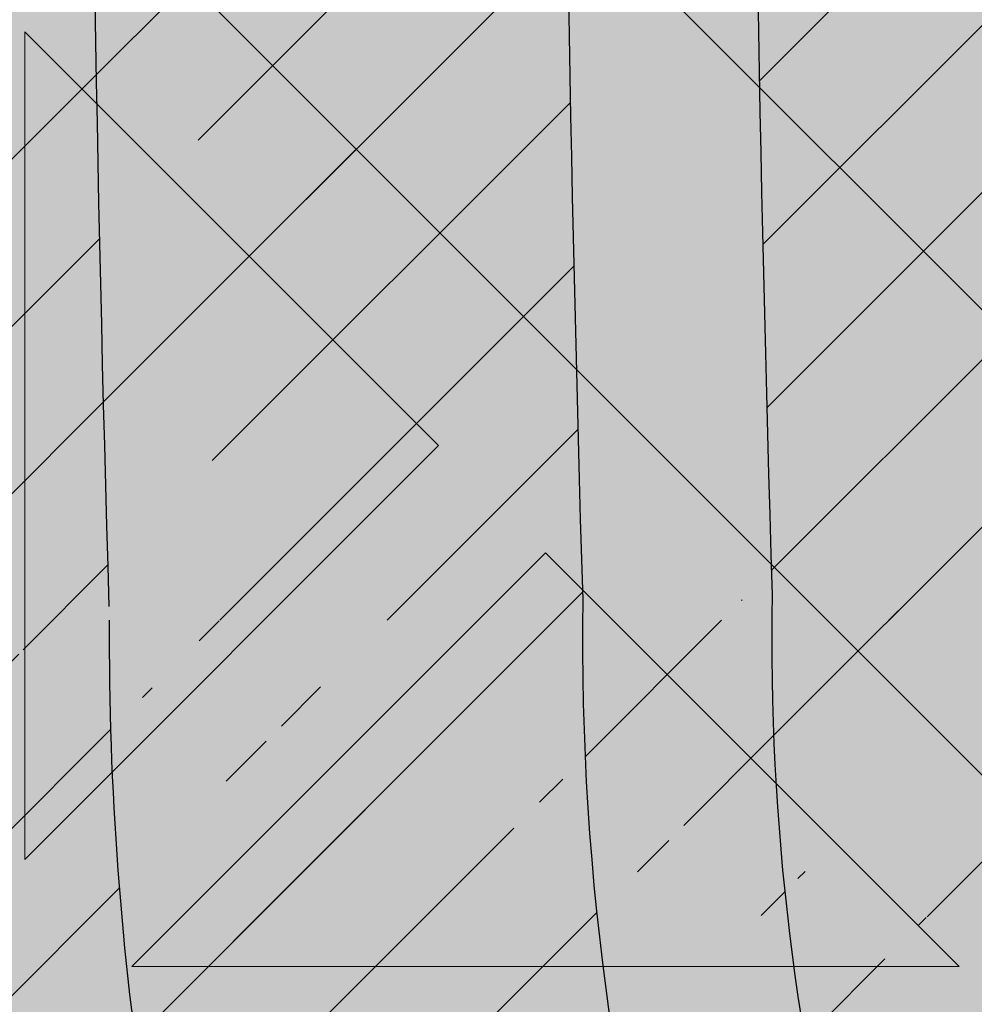
# Model space of a CAD drawing. Units: inches. Extents: x 844 to 2234, y 346 to 1084.
# Tile 11 of 93: x 1120.394 to 1122.002, y 691.183 to 692.842. Entities that reach past the tile are written whole.
import ezdxf

# ---------------------------------------------------------------- set-up
doc = ezdxf.new("R2010")
doc.units = ezdxf.units.IN
doc.header["$MEASUREMENT"] = 0
for name, color, linetype, lineweight in [('A-ANNO-DIMS', 2, 'Continuous', 18), ('furniture', 8, 'Continuous', 18), ('RA-AP-01$0$INT', 35, 'Continuous', 5)]:
    doc.layers.add(name, color=color, linetype=linetype, lineweight=lineweight)
doc.layers.add('RA-AP-01$0$FURN', color=3, linetype='Continuous')
doc.layers.add('RA-AP-01$0$WOOD', color=64, linetype='Continuous')
doc.styles.get("Standard").update_dxf_attribs({"font": 'arial.ttf'})
doc.dimstyles.get("Standard").update_dxf_attribs({"dimtxt": 6, "dimasz": 3, "dimexe": 0.18, "dimexo": 0.0625, "dimgap": 0.09, "dimtad": 0, "dimtih": 1, "dimtoh": 1, "dimdec": 1, "dimzin": 0, "dimdsep": 46, "dimlunit": 3, "dimtxsty": 'Standard', "dimblk": 'ARCHTICK', "dimcen": 0.09, "dimadec": 0, "dimazin": 0, "dimtfac": 1, "dimtdec": 1, "dimtofl": 0, "dimtmove": 0, "dimatfit": 3, "dimfxl": 1, "dimtolj": 1, "dimtzin": 0, "dimarcsym": 0})

# ---------------------------------------------------------------- blocks, each defined once
blk = doc.blocks.new('A$C18D01794')
at = {"layer": 'RA-AP-01$0$INT'}
h = blk.add_hatch(color=256, dxfattribs=at)
h.paths.add_polyline_path([(4.585917135068449, -6.356712009588271), (4.555206456959269, -6.35671200958746), (4.555206456959137, -6.387422687716308), (4.874495778835233, -6.706712009592356), (4.90520645695423, -6.676001331474049)])
h.paths.add_polyline_path([(5.255206456948813, -6.387422687716306), (5.255206456948682, -6.356712009605972), (5.224495778822613, -6.356712009605161), (4.905206456953498, -6.676001331474273), (4.935917135072151, -6.706712009592924)])
h.paths.add_polyline_path([(4.935917135072559, -6.706712009592068), (4.905206456953564, -6.737422687710376), (5.255206456951813, -7.087422687708613), (5.255206456951549, -7.026001331471008)])
h.paths.add_polyline_path([(4.555206456956399, -7.026001331471013), (4.555206456956134, -7.087422687708616), (4.905206456953821, -6.737422687710943), (4.874495778835166, -6.70671200959229)])
h = blk.add_hatch(color=256, dxfattribs=at)
h.paths.add_polyline_path([(4.585917135068448, -6.356712009588273), (4.614201406330596, -6.356712009589021), (4.668846067270487, -6.411356670531338), (4.723490728212344, -6.356712009591912), (4.771774999457151, -6.35671200959319), (4.826419660396886, -6.411356670535356), (4.862780050090322, -6.374996280843536), (4.844495778842715, -6.356712009595112), (4.862780050090411, -6.356712009595595), (4.905206456960182, -6.399138416468211), (4.947632863832445, -6.356712009597838), (4.965917135079675, -6.356712009598322), (4.947632863831759, -6.374996280845421), (4.983993253523576, -6.411356670538857), (5.038637914464627, -6.356712009600247), (5.08692218571208, -6.356712009601523), (5.141566846649976, -6.411356670541852), (5.196211507589851, -6.356712009604411), (5.224495778822615, -6.356712009605161), (4.905206456953975, -6.676001331473793)])
h.paths.add_polyline_path([(4.895206456956031, -6.637717060225675), (4.895206456958921, -6.528427738347902), (4.840561796018589, -6.583072399285802)], flags=16)
h.paths.add_polyline_path([(4.915206456955638, -6.637717060226121), (4.969851117895509, -6.583072399288678), (4.915206456957609, -6.528427738348344)], flags=16)
h.paths.add_polyline_path([(4.826419660395175, -6.568930263661755), (4.881064321335613, -6.514285602723745), (4.771774999456703, -6.514285602720857)], flags=16)
h.paths.add_polyline_path([(4.983993253519558, -6.568930263665262), (5.038637914460456, -6.514285602726792), (4.929348592581548, -6.514285602724816)], flags=16)
h.paths.add_polyline_path([(4.881064321336025, -6.494285602723742), (4.826419660397532, -6.439640941782821), (4.771774999457062, -6.494285602720859)], flags=16)
h.paths.add_polyline_path([(4.929348592582019, -6.494285602724817), (5.038637914460982, -6.494285602726792), (4.983993253522945, -6.439640941786327)], flags=16)
h.paths.add_polyline_path([(4.895206456960191, -6.480143467100443), (4.895206456962115, -6.407422687715913), (4.876922185715016, -6.389138416467584), (4.840561796021581, -6.425498806159401)], flags=16)
h.paths.add_polyline_path([(4.915206456958487, -6.480143467100889), (4.969851117899527, -6.425498806162279), (4.933490728206909, -6.389138416468043), (4.9152064569598, -6.40742268771434)], flags=16)
h.paths.add_polyline_path([(4.757632863832376, -6.480143467096812), (4.812277524772842, -6.425498806158772), (4.757632863834348, -6.370854145217844)], flags=16)
h.paths.add_polyline_path([(4.737632863832376, -6.480143467096286), (4.737632863834348, -6.370854145217375), (4.682988202893906, -6.425498806155385)], flags=16)
h.paths.add_polyline_path([(5.05278005008503, -6.480143467103376), (5.052780050087917, -6.370854145224413), (4.998135389146995, -6.425498806162908)], flags=16)
h.paths.add_polyline_path([(5.072780050085024, -6.480143467103744), (5.127424711025931, -6.42549880616527), (5.072780050087916, -6.370854145224832)], flags=16)
h.paths.add_polyline_path([(4.935917135072783, -6.706712009592292), (5.255206456948811, -6.387422687716309), (5.255206456948932, -6.415706958964177), (5.200561796010279, -6.470351619902839), (5.255206456949403, -6.524996280841948), (5.25520645694961, -6.5732805520894), (5.200561796009787, -6.627925213029239), (5.236922185702417, -6.664285602721864), (5.255206456949919, -6.646001331474357), (5.255206456949998, -6.664285602721898), (5.212780050078687, -6.706712009592262), (5.25520645695036, -6.749138416463932), (5.255206456950438, -6.767422687711313), (5.236922185702424, -6.749138416463297), (5.200561796009796, -6.785498806155928), (5.255206456950753, -6.840143467096874), (5.25520645695096, -6.888427738341682), (5.200561796010322, -6.943072399282328), (5.255206456951428, -6.997717060223427), (5.255206456951547, -7.026001331471006)])
h.paths.add_polyline_path([(5.042988202883395, -6.785498806155427), (5.097632863823085, -6.840143467095101), (5.097632863822622, -6.730854145216193)], flags=16)
h.paths.add_polyline_path([(5.028846067259663, -6.771356670531693), (5.083490728198774, -6.716712009592573), (4.974201406321001, -6.716712009593042)], flags=16)
h.paths.add_polyline_path([(5.117632863823087, -6.840143467095186), (5.172277524762331, -6.785498806155926), (5.11763286382262, -6.730854145216225)], flags=16)
h.paths.add_polyline_path([(5.08349072819877, -6.696712009593886), (5.028846067259652, -6.642067348654775), (4.974201406320998, -6.696712009593438)], flags=16)
h.paths.add_polyline_path([(5.131774999446817, -6.854285602718917), (5.186419660386065, -6.799640941779662), (5.241064321325782, -6.854285602719365)], flags=17)
h.paths.add_polyline_path([(5.131774999446228, -6.716712009592374), (5.186419660386065, -6.771356670532194), (5.222780050079488, -6.734996280838764), (5.204495778832781, -6.716712009592063)], flags=16)
h.paths.add_polyline_path([(5.097632863822613, -6.682569873970264), (5.097632863823061, -6.573280552091354), (5.042988202883383, -6.627925213031044)], flags=16)
h.paths.add_polyline_path([(5.131774999446899, -6.874285602718915), (5.241064321325809, -6.874285602719364), (5.186419660386591, -6.928930263658598)], flags=17)
h.paths.add_polyline_path([(5.131774999446226, -6.696712009594078), (5.204495778830767, -6.696712009594374), (5.22278005007868, -6.67842773834687), (5.186419660386049, -6.642067348654249)], flags=16)
h.paths.add_polyline_path([(5.11763286382262, -6.682569873970225), (5.17227752476232, -6.627925213030515), (5.117632863823064, -6.573280552091267)], flags=16)
h.paths.add_polyline_path([(5.186419660386069, -6.613783077405491), (5.241064321325754, -6.559138416465795), (5.131774999446791, -6.559138416466263)], flags=16)
h.paths.add_polyline_path([(5.131774999446872, -6.539138416466263), (5.24106432132578, -6.539138416465794), (5.186419660386554, -6.484493755526573)], flags=16)
h.paths.add_polyline_path([(5.255206456951811, -7.08742268770861), (5.255206456951895, -7.106712009588038), (4.555206456956052, -7.106712009588038), (4.555206456956136, -7.087422687708617), (4.905206456953973, -6.737422687710788)])
h.paths.add_polyline_path([(4.983993253513404, -6.8444937555241), (4.92934859257295, -6.899138416462108), (5.03863791445186, -6.899138416465014)], flags=16)
h.paths.add_polyline_path([(4.969851117889988, -6.83035161990006), (4.915206456952556, -6.775706958960171), (4.915206456949648, -6.884996280837944)], flags=16)
h.paths.add_polyline_path([(4.929348592572535, -6.919138416462105), (4.983993253511019, -6.973783077403037), (5.038637914451496, -6.919138416465012)], flags=16)
h.paths.add_polyline_path([(5.052780050074912, -6.93328055208906), (4.998135389134438, -6.987925213027088), (5.052780050072919, -7.042569873968025)], flags=16)
h.paths.add_polyline_path([(5.07278005007491, -6.933280552089588), (5.072780050072918, -7.042569873968497), (5.127424711013374, -6.987925213030498)], flags=16)
h.paths.add_polyline_path([(4.89520645695295, -6.775706958959721), (4.840561796013067, -6.830351619897157), (4.895206456950961, -6.884996280837494)], flags=16)
h.paths.add_polyline_path([(4.915206456948365, -6.933280552085403), (4.915206456946434, -7.006001331471951), (4.933490728192729, -7.024285602719066), (4.969851117886972, -6.987925213026453)], flags=16)
h.paths.add_polyline_path([(4.881064321327021, -6.899138416461022), (4.82641966038902, -6.84449375552057), (4.771774999448108, -6.899138416459029)], flags=16)
h.paths.add_polyline_path([(4.895206456950073, -6.933280552084951), (4.840561796009022, -6.987925213023558), (4.876922185700835, -7.024285602716997), (4.895206456948749, -7.006001331469487)], flags=16)
h.paths.add_polyline_path([(4.983993253510392, -7.0020673486505), (4.947632863816944, -7.038427738342319), (4.965917135064043, -7.05671200959023), (5.038637914448995, -7.056712009591555)], flags=16)
h.paths.add_polyline_path([(4.881064321326543, -6.91913841646102), (4.771774999447578, -6.919138416459031), (4.826419660385607, -6.973783077399508)], flags=16)
h.paths.add_polyline_path([(4.905206456946447, -7.014285602717636), (4.862780050074785, -7.056712009588352), (4.947632863816685, -7.056712009589775)], flags=16)
h.paths.add_polyline_path([(5.14156684663679, -7.002067348654549), (5.086922185696452, -7.056712009592438), (5.196211507574223, -7.056712009594425)], flags=16)
h.paths.add_polyline_path([(4.8264196603837, -7.002067348646972), (4.771774999442643, -7.056712009585575), (4.8444957788276, -7.056712009587508), (4.862780050075511, -7.038427738340416)], flags=16)
h.paths.add_polyline_path([(4.812277524760289, -6.98792521302292), (4.757632863822258, -6.933280552082447), (4.757632863819352, -7.042569873961408)], flags=16)
h.paths.add_polyline_path([(4.73763286382226, -6.933280552082079), (4.682988202881349, -6.987925213020536), (4.737632863819352, -7.04256987396099)], flags=16)
h.paths.add_polyline_path([(4.723490728195188, -7.056712009584289), (4.668846067257299, -7.002067348643949), (4.614201406317417, -7.056712009581383)], flags=16)
h.paths.add_polyline_path([(4.597632863829262, -6.706712009592262), (4.555206456957951, -6.664285602721896), (4.555206456958029, -6.646001331474357), (4.573490728205535, -6.664285602721864), (4.609851117898167, -6.627925213029238), (4.555206456958338, -6.573280552089402), (4.555206456958546, -6.524996280841952), (4.60985111789767, -6.470351619902839), (4.555206456959015, -6.415706958964177), (4.555206456959138, -6.387422687716309), (4.874495778835167, -6.70671200959229), (4.5552064569564, -7.026001331471015), (4.555206456956523, -6.997717060223433), (4.609851117897629, -6.94307239928233), (4.555206456956988, -6.888427738341681), (4.555206456957198, -6.840143467096881), (4.609851117898153, -6.78549880615593), (4.573490728205528, -6.749138416463297), (4.555206456957507, -6.76742268771132), (4.555206456957585, -6.749138416463933)])
h.paths.add_polyline_path([(4.712780050085332, -6.730854145216195), (4.712780050084863, -6.840143467095105), (4.767424711024555, -6.785498806155427)], flags=16)
h.paths.add_polyline_path([(4.726922185709173, -6.716712009592573), (4.781566846648288, -6.771356670531693), (4.836211507586949, -6.716712009593043)], flags=16)
h.paths.add_polyline_path([(4.692780050085327, -6.730854145216225), (4.638135389145619, -6.785498806155928), (4.692780050084865, -6.840143467095185)], flags=16)
h.paths.add_polyline_path([(4.726922185709182, -6.696712009593886), (4.836211507586949, -6.696712009593436), (4.7815668466483, -6.642067348654773)], flags=16)
h.paths.add_polyline_path([(4.678637914461726, -6.71671200959237), (4.605917135075169, -6.716712009592063), (4.587632863828464, -6.734996280838766), (4.623993253521887, -6.771356670532195)], flags=16)
h.paths.add_polyline_path([(4.712780050085336, -6.68256987397026), (4.767424711024568, -6.627925213031042), (4.71278005008489, -6.573280552091352)], flags=16)
h.paths.add_polyline_path([(4.678637914461726, -6.696712009594076), (4.623993253521899, -6.642067348654247), (4.587632863829271, -6.67842773834687), (4.605917135077185, -6.696712009594376)], flags=16)
h.paths.add_polyline_path([(4.692780050085336, -6.682569873970228), (4.692780050084889, -6.573280552091267), (4.638135389145632, -6.627925213030515)], flags=16)
h.paths.add_polyline_path([(4.623993253521885, -6.799640941779662), (4.678637914461131, -6.854285602718915), (4.56934859258217, -6.854285602719365)], flags=17)
h.paths.add_polyline_path([(4.623993253521901, -6.613783077405509), (4.678637914461158, -6.559138416466263), (4.569348592582195, -6.559138416465795)], flags=16)
h.paths.add_polyline_path([(4.678637914461051, -6.874285602718915), (4.623993253521361, -6.928930263658598), (4.569348592582143, -6.874285602719364)], flags=17)
h.paths.add_polyline_path([(4.678637914461076, -6.539138416466263), (4.623993253521399, -6.484493755526573), (4.569348592582167, -6.539138416465796)], flags=16)
h = blk.add_hatch(color=256, dxfattribs=at)
h.paths.add_polyline_path([(4.781566846647504, -6.771356670530272), (4.836211507586161, -6.716712009591613), (4.726922185708388, -6.716712009591159)])
h.paths.add_polyline_path([(4.836211507586161, -6.696712009592008), (4.781566846647504, -6.642067348653354), (4.726922185708388, -6.69671200959247)])
h.paths.add_polyline_path([(4.76742471102377, -6.627925213029623), (4.712780050084083, -6.57328055208994), (4.712780050084542, -6.68256987396885)])
h.paths.add_polyline_path([(4.692780050084544, -6.682569873968819), (4.692780050084084, -6.573280552089856), (4.638135389144834, -6.627925213029111)])
h.paths.add_polyline_path([(4.678637914460932, -6.696712009592669), (4.623993253521102, -6.642067348652844), (4.587632863827676, -6.678427738346266), (4.605917135074382, -6.696712009592973)])
h.paths.add_polyline_path([(4.573490728204743, -6.664285602721736), (4.60985111789737, -6.627925213029108), (4.555206456957541, -6.573280552089279), (4.555206456957237, -6.646001331474231)])
h.paths.add_polyline_path([(4.623993253521098, -6.613783077405377), (4.67863791446035, -6.559138416466126), (4.56934859258139, -6.559138416465669)])
h.paths.add_polyline_path([(4.678637914460275, -6.539138416466126), (4.623993253520583, -6.48449375552644), (4.56934859258136, -6.539138416465672)])
h.paths.add_polyline_path([(4.609851117896854, -6.470351619902707), (4.555206456958196, -6.415706958964051), (4.555206456957738, -6.524996280841822)])
h.paths.add_polyline_path([(4.597632863828475, -6.706712009592775), (4.555206456957283, -6.664285602721582), (4.555206456956805, -6.749138416463489)])
h.paths.add_polyline_path([(4.678637914460932, -6.716712009590963), (4.605917135076396, -6.71671200959066), (4.587632863828479, -6.734996280838164), (4.623993253521104, -6.771356670530792)])
h.paths.add_polyline_path([(4.692780050084091, -6.840143467093776), (4.692780050084548, -6.730854145214809), (4.638135389144834, -6.785498806154524)])
h.paths.add_polyline_path([(4.767424711023772, -6.785498806154004), (4.712780050084545, -6.730854145214786), (4.712780050084089, -6.840143467093692)])
h.paths.add_polyline_path([(4.67863791446036, -6.854285602718778), (4.623993253521105, -6.799640941779527), (4.569348592581399, -6.854285602719237)])
h.paths.add_polyline_path([(4.609851117897371, -6.785498806155798), (4.573490728204743, -6.74913841646317), (4.555206456957237, -6.767422687710675), (4.555206456957548, -6.840143467095629)])
h.paths.add_polyline_path([(4.623993253520596, -6.928930263658465), (4.67863791446028, -6.874285602718778), (4.569348592581367, -6.874285602719238)])
h.paths.add_polyline_path([(4.609851117896867, -6.943072399282199), (4.555206456957749, -6.888427738343082), (4.55520645695821, -6.997717060220857)])
for p, q in [((4.874495778835167, -6.70671200959229), (4.555206456956399, -7.026001331471013)), ((4.726922185709178, -6.716712009592574), (4.836211507586949, -6.716712009593042)), ((4.72692218570918, -6.716712009592578), (4.781566846648288, -6.771356670531693)), ((4.836211507586949, -6.716712009593042), (4.781566846648288, -6.771356670531693)), ((4.712780050084865, -6.840143467095105), (4.71278005008533, -6.730854145216195)), ((4.71278005008533, -6.730854145216195), (4.767424711024555, -6.785498806155425)), ((4.905206456953975, -6.737422687710788), (4.555206456956136, -7.087422687708617)), ((4.767424711024554, -6.785498806155427), (4.712780050084865, -6.840143467095105))]:
    blk.add_line(p, q, dxfattribs=at)
blk = doc.blocks.new('A$C32926AE1')
at = {"layer": 'RA-AP-01$0$FURN'}
h = blk.add_hatch(dxfattribs=at)
h.set_pattern_fill('ANSI31', color=256, scale=0.1, style=0)
h.set_pattern_definition([(45, (0, 0), (-0.0088388347648318, 0.0088388347648318), [])])
edge = h.paths.add_edge_path(flags=16)
edge.add_arc((4.904771284329206, 4.246793130718756), 0.2603971832811541, 75.22398030683196, 104.7760196931204)
edge.add_arc((4.904771284329206, 4.246793130718756), 0.2603971832811541, 75.223980306832, 104.77601969312039, ccw=False)
edge = h.paths.add_edge_path(flags=16)
edge.add_arc((4.904771284329206, 4.067062675376612), 0.2603971832811541, 255.2239803068796, 284.776019693168)
edge.add_arc((4.904771284329206, 4.067062675376612), 0.2603971832811541, 255.22398030687958, 284.77601969316805, ccw=False)
edge = h.paths.add_edge_path(flags=0)
edge.add_arc((4.904771284329206, 4.067062675376612), 0.2603971832811541, 255.2239803068796, 284.776019693168)
edge.add_arc((4.904771284329206, 4.067062675376612), 0.2603971832811541, 255.22398030687958, 284.77601969316805, ccw=False)
edge = h.paths.add_edge_path(flags=0)
edge.add_arc((4.904771284329206, 4.067062675376612), 0.2603971832811541, 255.2239803068796, 284.776019693168)
edge.add_arc((4.904771284329206, 4.067062675376612), 0.2603971832811541, 255.22398030687958, 284.77601969316805, ccw=False)
edge = h.paths.add_edge_path()
edge.add_arc((4.604388392048174, 4.588829985554312), 0.1599999999999918, 342.3781640246255, 354.4317409793762)
edge.add_arc((5.090145208887507, 4.43216705527679), 0.3503971832811637, 162.0091218307731, 180.3186872093483)
edge.add_arc((5.205154176610243, 4.588829985554953), 0.1599999999999917, 185.5682590208461, 197.6218359767349)
edge.add_arc((4.904771284329229, 4.246793130718735), 0.3503971832811761, 72.00912183053516, 107.9908781690354)
edge.add_arc((9.535952835716557, 4.28682295566602), 4.798342501046485, 178.2875002453811, 181.5576802719453)
edge.add_arc((4.719397359771122, 4.43216705527679), 0.3503971832811637, 359.6813127906516, 377.9908781692269)
edge.add_arc((9.535967292294904, 4.286822350292874), 4.778371420254705, 178.2965938931842, 181.5667745797229)
edge.add_arc((4.719397359771122, 4.43216705527679), 0.3303971832811637, 359.6813127906516, 377.9908781692269)
edge.add_arc((0.2735752763637294, 4.286822350292874), 4.7783714202547, 358.4332254202771, 361.7034061068158)
edge.add_arc((5.061434214606998, 4.732549947558029), 0.1600000000000254, 252.3781640250584, 264.4317409792362)
edge.add_arc((4.748108354051257, 4.732549947558012), 0.1600000000000541, 275.5682590208426, 287.6218359759532)
edge.add_arc((4.604388392048115, 4.588829985554317), 0.1800000000000505, 342.3567572500182, 349.3735009646207)
edge.add_arc((5.205154176610254, 4.588829985554976), 0.1800000000000069, 190.6264990356027, 197.6432427513933)
edge.add_arc((5.061434214607106, 4.732549947558013), 0.1800000000000424, 252.3567572496606, 259.3735009644582)
edge.add_arc((4.904771284329208, 4.246793130718737), 0.3303971832811676, 71.99844483668534, 108.0015551637021)
edge.add_arc((4.748108354051414, 4.732549947558045), 0.1800000000000547, 280.6264990355479, 287.6432427495938)
edge.add_arc((5.090145208887514, 4.432167055276789), 0.2803971832811691, 162.8706300666893, 180.816523289902)
edge.add_arc((4.719397359771136, 4.432167055276689), 0.2803971832811534, 359.183476710103, 377.1293699333214)
edge.add_arc((4.904771284329222, 4.246793130718737), 0.2803971832811769, 72.87063006672916, 107.1293699332334)
edge.add_arc((5.090145208887522, 4.432167055276788), 0.2603971832811776, 165.2239803068007, 180.9953123810312)
edge.add_arc((4.719397359771141, 4.432167055276699), 0.2603971832811458, 359.0046876189768, 374.7760196932087)
edge.add_arc((5.090145208887507, 4.43216705527679), 0.3303971832811637, 162.0091218307731, 180.3186872093483)
edge.add_arc((9.53595427642584, 4.285015535491528), 4.728345371032053, 178.265043920078, 181.5679956281801)
edge.add_arc((0.2735882922327999, 4.285015535491582), 4.728345371032045, 358.4320043718193, 361.7349560799204)
edge.add_arc((9.535953591267507, 4.284458026472751), 4.708343996644348, 178.2573054306777, 181.5704995759608)
edge.add_arc((0.273588977391114, 4.284458026472785), 4.708343996644358, 358.4295004240388, 361.7426945693213)
edge.add_arc((0.2735889773911131, 4.029397779622582), 4.708343996644359, 358.2573054306787, 361.5704995759613)
edge.add_arc((9.535953591267518, 4.029397779622618), 4.708343996644359, 178.4295004240391, 181.7426945693223)
edge.add_arc((0.2735882922327901, 4.028840270603786), 4.728345371032054, 358.2650439200796, 361.5679956281808)
edge.add_arc((9.53595427642584, 4.028840270603841), 4.728345371032054, 178.4320043718199, 181.7349560799219)
edge.add_arc((0.2735752763637302, 4.027033455802493), 4.778371420254699, 358.2965938931842, 361.5667745797229)
edge.add_arc((4.719397359771122, 3.881688750818578), 0.3303971832811637, 342.0091218307731, 360.3186872093484)
edge.add_arc((5.090145208887507, 3.881688750818578), 0.3303971832811637, 179.6813127906516, 197.9908781692269)
edge.add_arc((9.535967292294904, 4.027033455802493), 4.778371420254705, 178.433225420277, 181.7034061068158)
edge.add_arc((4.719397359771122, 3.881688750818578), 0.3503971832811637, 342.0091218307731, 360.3186872093484)
edge.add_arc((9.53595283571655, 4.027032850429349), 4.79834250104648, 178.4423197280546, 181.7124997546188)
edge.add_arc((4.719397359771141, 3.881688750818669), 0.2603971832811458, 345.2239803067913, 360.9953123810232)
edge.add_arc((5.090145208887522, 3.88168875081858), 0.2603971832811776, 179.0046876189687, 194.7760196931993)
edge.add_arc((4.904771284329222, 4.067062675376631), 0.2803971832811769, 252.8706300667665, 287.1293699332708)
edge.add_arc((4.719397359771136, 3.881688750818678), 0.2803971832811534, 342.8706300666787, 360.8165232898969)
edge.add_arc((5.090145208887514, 3.881688750818579), 0.2803971832811691, 179.183476710098, 197.1293699333106)
edge.add_arc((4.748108354051414, 3.581305858537323), 0.1800000000000547, 72.3567572504062, 79.37350096445199)
edge.add_arc((4.904771284329208, 4.067062675376631), 0.3303971832811676, 251.9984448362979, 288.0015551633146)
edge.add_arc((5.061434214607106, 3.581305858537355), 0.1800000000000424, 100.6264990355418, 107.6432427503394)
edge.add_arc((5.205154176610254, 3.725025820540392), 0.1800000000000069, 162.3567572486066, 169.3735009643972)
edge.add_arc((4.604388392048115, 3.725025820541051), 0.1800000000000505, 10.62649903537925, 17.64324274998182)
edge.add_arc((4.748108354051257, 3.581305858537356), 0.1600000000000541, 72.37816402404681, 84.43174097915735)
edge.add_arc((4.904771284329229, 4.067062675376632), 0.3503971832811761, 252.0091218309645, 287.9908781694648)
edge.add_arc((5.061434214606998, 3.581305858537339), 0.1600000000000254, 95.56825902076373, 107.6218359749416)
edge.add_arc((5.205154176610243, 3.725025820540414), 0.1599999999999917, 162.3781640232651, 174.4317409791539)
edge.add_arc((5.090145208887507, 3.881688750818578), 0.3503971832811637, 179.6813127906516, 197.9908781692269)
edge.add_arc((4.604388392048174, 3.725025820541056), 0.1599999999999918, 5.568259020623824, 17.62183597537444)
edge.add_arc((0.2735897329420762, 4.28682295566602), 4.798342501046482, 358.4423197280547, 361.7124997546188)
edge.add_arc((0.2735897329420691, 4.027032850429348), 4.798342501046489, 358.2875002453812, 361.5576802719453)
at = {"layer": 'RA-AP-01$0$WOOD'}
h = blk.add_hatch(color=256, dxfattribs=at)
h.dxf.hatch_style = 1
h.paths.add_polyline_path([(5.157430609644524, 4.573483066760929, -0.1009492694046607), (5.155401577623758, 4.593365984175333, -0.1842662638101597), (5.172249623284174, 4.638795604568598, 0.2056608120311276), (5.179560981299304, 4.661316324430096, 0.3614336704623542), (5.134352340494423, 4.706524965234944, 0.2056608120311297), (5.111831620632933, 4.699213607219793, -0.1842662638101113), (5.066402000239693, 4.682365561559342, -0.1055311479399994), (5.045656153913092, 4.68467289944697, 0.1567636581983829), (4.763886414745334, 4.684672899446966, -0.1055311479399895), (4.743140568418733, 4.68236556155934, -0.1842662638100833), (4.6977109480255, 4.69921360721979, 0.2056608120302612), (4.675190228164109, 4.706524965234949, 0.3614336704708441), (4.629981587358889, 4.66131632442871, 0.2056608120245944), (4.637292945374126, 4.638795604567974, -0.1842662638101024), (4.654140991034615, 4.59336598417475, -0.1009492694055169), (4.652111959013835, 4.573483066760181, 0.021410119221476), (4.629748025606143, 4.156712009541676, 0.0214101192214795), (4.652111959013809, 3.739940952323101, -0.1009492694059586), (4.654140991034615, 3.720058034908448, -0.1842662638100975), (4.637292945374126, 3.674628414515226, 0.2056608120245705), (4.629981587358889, 3.652107694654492, 0.3614336704708879), (4.675190228164113, 3.606899053848249, 0.2056608120302384), (4.697710948025501, 3.614210411863408, -0.1842662638100995), (4.743140568418738, 3.63105845752386, -0.1055311479402541), (4.763886414745388, 3.628751119636215, 0.1567636581983776), (5.045656153913137, 3.628751119636244, -0.1055311479397538), (5.066402000239692, 3.631058457523857, -0.1842662638101067), (5.111831620632931, 3.614210411863407, 0.2056608120310924), (5.134352340494417, 3.606899053848256, 0.3614336704624001), (5.179560981299307, 3.652107694653103, 0.2056608120311314), (5.172249623284175, 3.6746284145146, -0.1842662638101402), (5.155401577623758, 3.72005803490786, -0.1009492694051366), (5.15743060964455, 3.739940952322354, 0.0214101192215073), (5.179794543052287, 4.156712009541468, 0.0214101192215252)])
h.paths.add_polyline_path([(4.639748609479751, 4.156712009541513, 0.0213537860821624), (4.661970494867118, 3.741887061152232, -0.094075836301374), (4.664143710413708, 3.7196126951003, -0.1824818158568985), (4.644813765429836, 3.668037719127816, 0.2056608120245319), (4.639939526753007, 3.653023905887301, 0.3614336704710246), (4.676106439397173, 3.616856993242342, 0.2056608120302234), (4.691120252638095, 3.621731231919122, -0.1824818158602558), (4.742695228611606, 3.641061176902986, -0.1029891339458722), (4.766991894714349, 3.638256818950944, 0.156709409989566), (5.042550673941472, 3.638256818950105, -0.102989133958497), (5.066847340047078, 3.641061176902949, -0.1824818158594995), (5.118422316020358, 3.621731231919103, 0.2056608120311416), (5.133436129261316, 3.616856993242346, 0.3614336704621468), (5.169603041905217, 3.653023905886178, 0.2056608120310986), (5.164728803228477, 3.668037719127177, -0.1824818158565612), (5.145398858244737, 3.719612695099578, -0.0940758363009313), (5.147572073791232, 3.741887061151398, 0.0213537860822023), (5.169793959178681, 4.156712009541451, 0.0213537860822226), (5.147572073791203, 4.571536957931898, -0.0940758363005034), (5.145398858244737, 4.59381132398362, -0.1824818158565587), (5.164728803228476, 4.645386299956021, 0.2056608120311045), (5.169603041905216, 4.66040011319702, 0.3614336704621845), (5.133436129261313, 4.696567025840856, 0.2056608120310773), (5.118422316020359, 4.691692787164098, -0.182481815859508), (5.066847340047078, 4.67236284218025, -0.1029891339584606), (5.04255067394148, 4.675167200133092, 0.156709409989566), (4.766991894714357, 4.675167200132257, -0.1029891339458842), (4.742695228611611, 4.672362842180213, -0.1824818158602725), (4.691120252638095, 4.691692787164077, 0.2056608120302152), (4.676106439397174, 4.696567025840858, 0.3614336704710363), (4.639939526753005, 4.660400113195899, 0.2056608120245495), (4.644813765429837, 4.645386299955384, -0.1824818158568934), (4.664143710413708, 4.593811323982902, -0.0940758363009187), (4.661970494867149, 4.571536957931074, 0.021353786082177)], flags=16)
h.paths.add_polyline_path([(5.129794543052235, 4.432167055276933, -0.0141661062790638), (5.130152669293814, 4.156927903047693, -0.0141661062790647), (5.129794543052234, 3.881688750818433, -0.0785247771143638), (5.10979738006795, 3.755143611847103, 0.0945969212073497), (5.105408519571111, 3.717898134952927, 0.1043170707844957), (5.116074640131521, 3.670385395016088, 0.1043170707864965), (5.068561900193738, 3.681051515576561, 0.09459692119553), (5.031316423304057, 3.676662655080835, -0.1580239521427272), (4.778226145355827, 3.676662655080367, 0.0945969211986668), (4.740980668464973, 3.681051515576592, 0.1043170707882822), (4.693467928526415, 3.670385395015844, 0.1043170707867916), (4.704134049087309, 3.717898134953662, 0.0945969211972894), (4.69974518859162, 3.755143611844042, -0.0785247771163196), (4.679748025606343, 3.881688750818406, -0.0141661062790663), (4.679389899364763, 4.156927903047693, -0.0141661062790672), (4.679748025606343, 4.432167055276998, -0.0785247771163064), (4.699745188591625, 4.55871219425134, 0.094596921197333), (4.704134049087308, 4.595957671141738, 0.1043170707867205), (4.693467928526416, 4.643470411079523, 0.1043170707882628), (4.740980668464965, 4.632804290518776, 0.0945969211988114), (4.778226145355874, 4.637193151015016, -0.158023952142669), (5.031316423304015, 4.637193151014546, 0.0945969211956361), (5.068561900193736, 4.632804290518806, 0.1043170707864979), (5.11607464013152, 4.643470411079278, 0.1043170707844617), (5.105408519571112, 4.595957671142455, 0.0945969212074597), (5.109797380067959, 4.558712194248236, -0.0785247771143467)], flags=0)
h.paths.add_polyline_path([(5.119794532311105, 4.432259799204851, -0.0142000800617244), (5.120156169157484, 4.156927903047701, -0.0142000800617277), (5.119794532311105, 3.881596006890482, -0.0784894509520253), (5.100273383573699, 3.758192358677797, 0.0940138827242913), (5.095413455884425, 3.717477693979438, 0.0606271852308753), (5.099615656341024, 3.686844378806616, 0.0606271852322524), (5.068982341167493, 3.691046579263239, 0.0940138827010453), (5.028267676478798, 3.686186651576848, -0.1580706864508061), (4.781274892180912, 3.686186651576435, 0.0940138827026903), (4.740560227491556, 3.691046579263279, 0.0606271852339895), (4.709926912317155, 3.686844378806508, 0.0606271852329405), (4.714129112773991, 3.717477693980356, 0.094013882701304), (4.709269185087677, 3.758192358669163, -0.0784894509577193), (4.689748036347473, 3.881596006890469, -0.014200080061729), (4.689386399501094, 4.156927903047709, -0.0142000800617217), (4.689748036347473, 4.432259799204808, -0.078489450957724), (4.709269185087651, 4.555663447426125, 0.0940138827014585), (4.714129112773992, 4.596378112114996, 0.0606271852329731), (4.709926912317154, 4.62701142728886, 0.0606271852340196), (4.74056022749157, 4.622809226832087, 0.0940138827024997), (4.781274892180847, 4.627669154518912, -0.1580706864508359), (5.028267676478777, 4.627669154518526, 0.0940138827010946), (5.068982341167492, 4.622809226832129, 0.060627185232254), (5.099615656341024, 4.627011427288751, 0.0606271852308727), (5.095413455884425, 4.59637811211593, 0.0940138827241088), (5.100273383573675, 4.555663447417647, -0.0784894509520978)], flags=0)
h.paths.add_polyline_path([(5.06978912287499, 4.430218106756144, -0.014241683694547), (5.070173729147532, 4.156927903047672, -0.0142416836945458), (5.06978912287499, 3.883637699339223, -0.0800609523125196), (5.052662118612511, 3.773463122773442, 0.0526421978001116), (5.04590916754064, 3.740550867606997, 0.0526421977992423), (5.012996912374707, 3.73379791653534, -0.1583028414718258), (4.796545656286308, 3.73379791653451, 0.0526421978034211), (4.763633401117837, 3.740550867607021, 0.0526421978018622), (4.756880450045755, 3.773463122774558, -0.0800609523117106), (4.739753445783639, 3.883637699339268, -0.0142416836945435), (4.739368839511098, 4.156927903047671, -0.0142416836945477), (4.739753445783639, 4.430218106756155, -0.0800609523116345), (4.75688045004574, 4.540392683320762, 0.052642197801941), (4.763633401117837, 4.573304938488346, 0.0526421978035071), (4.796545656286361, 4.580057889560873, -0.1583028414717561), (5.012996912374669, 4.580057889560039, 0.0526421977993048), (5.04590916754064, 4.57330493848837, 0.0526421978002057), (5.052662118612529, 4.540392683321868, -0.080060952312477)], flags=0)
h.paths.add_polyline_path([(5.049789715110557, 4.43038092723357, -0.0143097550741839), (5.05018085590259, 4.156927903047715, -0.0143097550741854), (5.049789715110558, 3.883474878861827, -0.0800685599149176), (5.03362098255317, 3.779581877367999, 0.0306258898956367), (5.028241146483733, 3.758218888663947, 0.0306258898977031), (5.006878157778253, 3.75283905259408, -0.1583983521624096), (4.802664410878162, 3.752839052594731, 0.0306258898946014), (4.781301422174808, 3.758218888663924, 0.0306258898967912), (4.775921586105202, 3.779581877368794, -0.080068559914251), (4.759752853548071, 3.883474878861786, -0.0143097550741854), (4.759361712756037, 4.156927903047671, -0.0143097550741854), (4.759752853548071, 4.430380927233557, -0.0800685599142479), (4.775921586105193, 4.534273928726546, 0.0306258898968306), (4.781301422174808, 4.555636917431444, 0.0306258898945754), (4.802664410878143, 4.561016753500631, -0.1583983521624168), (5.006878157778244, 4.561016753501291, 0.0306258898977177), (5.028241146483733, 4.555636917431421, 0.0306258898958182), (5.03362098255321, 4.534273928727244, -0.080068559914796)], flags=0)
h.paths.add_polyline_path([(4.999766070382627, 4.428171244713864, -0.0143443147609634), (5.000198441819402, 4.156927903047689, -0.0143443147609612), (4.999766070382627, 3.885684561381556, -0.0784641635803329), (4.987356730658798, 3.799103304488872, -0.1506053783831347), (4.822185837999821, 3.79910330448882, -0.0784641635803318), (4.809776498276007, 3.885684561381509, -0.014344314760963), (4.809344126839227, 4.156927903047677, -0.0143443147609645), (4.809776498276007, 4.428171244713873, -0.0784641635803192), (4.822185837999822, 4.514752501606549, -0.1506053783831338), (4.987356730658798, 4.514752501606494, -0.078464163580285)], flags=0)
h.paths.add_polyline_path([(4.979755254238824, 4.42764379880488, -0.0143772539198268), (4.980205517789977, 4.156927903047693, -0.0143772539198275), (4.979755254238824, 3.886212007290489, -0.0689242507424422), (4.971183264704897, 3.815276770442801, -0.1296645318904179), (4.838359303953726, 3.815276770442746, -0.0689242507424186), (4.829787314419809, 3.886212007290419, -0.0143772539198292), (4.829337050868653, 4.156927903047653, -0.0143772539198325), (4.829787314419809, 4.427643798804946, -0.0689242507424211), (4.838359303953725, 4.498579035652621, -0.1296645318904187), (4.971183264704897, 4.498579035652565, -0.0689242507424401)], flags=0)
h = blk.add_hatch(color=256, dxfattribs=at)
h.dxf.hatch_style = 1
h.paths.add_polyline_path([(5.145398858244737, 4.59381132398362, -0.1824818158565616), (5.164728803228476, 4.645386299956021, 0.2056608120311045), (5.169603041905216, 4.66040011319702, 0.3614336704621845), (5.133436129261313, 4.696567025840856, 0.2056608120310773), (5.118422316020359, 4.691692787164098, -0.182481815859508), (5.066847340047078, 4.67236284218025, -0.1029891339584606), (5.04255067394148, 4.675167200133092, 0.156709409989566), (4.766991894714357, 4.675167200132257, -0.1029891339458842), (4.742695228611611, 4.672362842180213, -0.1824818158602725), (4.691120252638095, 4.691692787164077, 0.2056608120302152), (4.676106439397174, 4.696567025840858, 0.3614336704710363), (4.639939526753005, 4.660400113195899, 0.2056608120245495), (4.644813765429837, 4.645386299955384, -0.1824818158568934), (4.664143710413708, 4.593811323982902, -0.0940758363009187), (4.661970494867149, 4.571536957931074, 0.0213537860821772), (4.639748609479751, 4.156712009541507, 0.0213537860821625), (4.661970494867119, 3.741887061152226, -0.0940758363013071), (4.664143710413708, 3.719612695100309, -0.1824818158569294), (4.644813765429836, 3.668037719127816, 0.2056608120245319), (4.639939526753007, 3.653023905887301, 0.3614336704710246), (4.676106439397173, 3.616856993242342, 0.2056608120302234), (4.691120252638095, 3.621731231919122, -0.1824818158602558), (4.742695228611606, 3.641061176902986, -0.1029891339458722), (4.766991894714349, 3.638256818950944, 0.156709409989566), (5.042550673941472, 3.638256818950105, -0.102989133958497), (5.066847340047078, 3.641061176902949, -0.1824818158594995), (5.118422316020358, 3.621731231919103, 0.2056608120311416), (5.133436129261316, 3.616856993242346, 0.3614336704621468), (5.169603041905217, 3.653023905886178, 0.2056608120310986), (5.164728803228477, 3.668037719127177, -0.1824818158565612), (5.145398858244737, 3.719612695099578, -0.0940758363009313), (5.147572073791232, 3.741887061151398, 0.0213537860822023), (5.169793959178681, 4.156712009541451, 0.0213537860822226), (5.147572073791203, 4.571536957931898, -0.0940758363004996)])
h.paths.add_polyline_path([(5.109797380067958, 4.55871219424824, -0.0785247771143472), (5.129794543052234, 4.432167055276936, -0.0141661062790644), (5.130152669293814, 4.156927903047685, -0.014166106279066), (5.129794543052234, 3.881688750818401, -0.0785247771143517), (5.109797380067946, 3.755143611847092, 0.0945969212073132), (5.105408519571111, 3.717898134952929, 0.1043170707844995), (5.116074640131521, 3.670385395016088, 0.1043170707864965), (5.068561900193738, 3.681051515576561, 0.09459692119553), (5.031316423304057, 3.676662655080835, -0.1580239521427272), (4.778226145355827, 3.676662655080367, 0.0945969211986668), (4.740980668464973, 3.681051515576592, 0.1043170707882822), (4.693467928526415, 3.670385395015844, 0.1043170707867916), (4.704134049087309, 3.717898134953662, 0.0945969211972894), (4.69974518859162, 3.755143611844042, -0.0785247771163196), (4.679748025606343, 3.881688750818406, -0.0141661062790663), (4.679389899364763, 4.156927903047693, -0.0141661062790672), (4.679748025606343, 4.432167055276998, -0.0785247771163064), (4.699745188591625, 4.55871219425134, 0.094596921197333), (4.704134049087308, 4.595957671141738, 0.1043170707867205), (4.693467928526416, 4.643470411079523, 0.1043170707882628), (4.740980668464965, 4.632804290518776, 0.0945969211988114), (4.778226145355874, 4.637193151015016, -0.158023952142669), (5.031316423304015, 4.637193151014546, 0.0945969211956361), (5.068561900193736, 4.632804290518806, 0.1043170707864979), (5.11607464013152, 4.643470411079278, 0.1043170707844617), (5.105408519571112, 4.595957671142455, 0.0945969212074504)], flags=16)
h.paths.add_polyline_path([(5.100273383573655, 4.55566344741771, -0.0784894509521388), (5.119794532311105, 4.432259799204852, -0.0142000800617252), (5.120156169157484, 4.156927903047686, -0.014200080061726), (5.119794532311105, 3.881596006890502, -0.0784894509520446), (5.100273383573696, 3.758192358677786, 0.0940138827242721), (5.095413455884425, 3.717477693979436, 0.0606271852308692), (5.099615656341024, 3.686844378806616, 0.0606271852322522), (5.068982341167493, 3.691046579263239, 0.0940138827010453), (5.028267676478798, 3.686186651576848, -0.1580706864508061), (4.781274892180912, 3.686186651576435, 0.0940138827026903), (4.740560227491556, 3.691046579263279, 0.0606271852339895), (4.709926912317155, 3.686844378806508, 0.0606271852329405), (4.714129112773991, 3.717477693980356, 0.094013882701304), (4.709269185087677, 3.758192358669163, -0.0784894509577193), (4.689748036347473, 3.881596006890469, -0.014200080061729), (4.689386399501094, 4.156927903047709, -0.0142000800617217), (4.689748036347473, 4.432259799204808, -0.078489450957724), (4.709269185087651, 4.555663447426125, 0.0940138827014585), (4.714129112773992, 4.596378112114996, 0.0606271852329731), (4.709926912317154, 4.62701142728886, 0.0606271852340196), (4.74056022749157, 4.622809226832087, 0.0940138827024997), (4.781274892180847, 4.627669154518912, -0.1580706864508359), (5.028267676478777, 4.627669154518526, 0.0940138827010946), (5.068982341167492, 4.622809226832129, 0.060627185232254), (5.099615656341024, 4.627011427288751, 0.0606271852308727), (5.095413455884425, 4.59637811211593, 0.094013882723957)], flags=0)
h.paths.add_polyline_path([(5.04590916754064, 4.57330493848837, 0.0526421978002057), (5.052662118612529, 4.540392683321868, -0.0800609523124783), (5.06978912287499, 4.430218106756142, -0.0142416836945469), (5.070173729147532, 4.156927903047672, -0.0142416836945458), (5.06978912287499, 3.883637699339223, -0.0800609523125196), (5.052662118612511, 3.773463122773442, 0.0526421978001116), (5.04590916754064, 3.740550867606997, 0.0526421977992423), (5.012996912374707, 3.73379791653534, -0.1583028414718258), (4.796545656286308, 3.73379791653451, 0.0526421978034211), (4.763633401117837, 3.740550867607021, 0.0526421978018622), (4.756880450045755, 3.773463122774558, -0.0800609523117106), (4.739753445783639, 3.883637699339268, -0.0142416836945435), (4.739368839511098, 4.156927903047671, -0.0142416836945477), (4.739753445783639, 4.430218106756155, -0.0800609523116345), (4.75688045004574, 4.540392683320762, 0.052642197801941), (4.763633401117837, 4.573304938488346, 0.0526421978035071), (4.796545656286361, 4.580057889560873, -0.1583028414717561), (5.012996912374669, 4.580057889560039, 0.0526421977993048)], flags=0)
h.paths.add_polyline_path([(5.028241146483733, 4.555636917431422, 0.0306258898956949), (5.033620982553182, 4.534273928727329, -0.0800685599148649), (5.049789715110557, 4.430380927233569, -0.0143097550741839), (5.05018085590259, 4.156927903047715, -0.0143097550741854), (5.049789715110558, 3.883474878861827, -0.0800685599149176), (5.03362098255317, 3.779581877367999, 0.0306258898956367), (5.028241146483733, 3.758218888663947, 0.0306258898977031), (5.006878157778253, 3.75283905259408, -0.1583983521624096), (4.802664410878162, 3.752839052594731, 0.0306258898946014), (4.781301422174808, 3.758218888663924, 0.0306258898967912), (4.775921586105202, 3.779581877368794, -0.080068559914251), (4.759752853548071, 3.883474878861786, -0.0143097550741854), (4.759361712756037, 4.156927903047671, -0.0143097550741854), (4.759752853548071, 4.430380927233557, -0.0800685599142479), (4.775921586105193, 4.534273928726546, 0.0306258898968306), (4.781301422174808, 4.555636917431444, 0.0306258898945754), (4.802664410878143, 4.561016753500631, -0.1583983521624168), (5.006878157778244, 4.561016753501291, 0.0306258898977174)], flags=0)
h.paths.add_polyline_path([(4.987356730658798, 4.514752501606494, -0.0784641635803018), (4.999766070382627, 4.428171244713845, -0.0143443147609637), (5.000198441819402, 4.156927903047665, -0.0143443147609622), (4.999766070382628, 3.885684561381514, -0.0784641635802952), (4.987356730658797, 3.799103304488872, -0.1506053783831338), (4.822185837999821, 3.799103304488819, -0.0784641635803342), (4.809776498276007, 3.885684561381512, -0.0143443147609628), (4.809344126839227, 4.156927903047676, -0.0143443147609646), (4.809776498276007, 4.428171244713873, -0.0784641635803192), (4.822185837999822, 4.514752501606549, -0.1506053783831338)], flags=0)
h.paths.add_polyline_path([(4.971183264704897, 4.498579035652566, -0.0689242507424384), (4.979755254238824, 4.427643798804883, -0.0143772539198276), (4.980205517789977, 4.15692790304768, -0.0143772539198258), (4.979755254238823, 3.88621200729051, -0.0689242507424628), (4.971183264704897, 3.815276770442801, -0.129664531890417), (4.838359303953726, 3.815276770442746, -0.0689242507424186), (4.829787314419809, 3.886212007290419, -0.0143772539198292), (4.829337050868653, 4.156927903047653, -0.0143772539198325), (4.829787314419809, 4.427643798804946, -0.0689242507424211), (4.838359303953725, 4.498579035652621, -0.1296645318904187)], flags=0)
h = blk.add_hatch(dxfattribs=at)
h.set_pattern_fill('ANSI31', color=256, scale=0.05, style=0)
h.set_pattern_definition([(45, (0, 0), (-0.0044194173824159, 0.0044194173824159), [])])
h.paths.add_polyline_path([(5.130152669293814, 4.156927903047704, 0.0141661062790657), (5.129794543052234, 4.432167055276982, 0.0777827904001433), (5.110168979996553, 4.557559993161921, -0.0976515123401879), (5.105408519571111, 4.595957671142454, -0.1043170707844687), (5.116074640131522, 4.64347041107928), (5.099615656341024, 4.627011427288751, 0.0606271852308727), (5.095413455884425, 4.59637811211593, 0.0940138827241088), (5.100273383573675, 4.555663447417647, -0.0784894509520972), (5.119794532311105, 4.432259799204852, -0.0142000800617252), (5.120156169157484, 4.156927903047686, -0.014200080061726), (5.119794532311105, 3.881596006890502, -0.0784894509520446), (5.100273383573696, 3.758192358677786, 0.0940138827242721), (5.095413455884425, 3.717477693979436, 0.0606271852308692), (5.099615656341024, 3.686844378806616), (5.116074640131519, 3.67038539501609, -0.1043170707844594), (5.105408519571112, 3.717898134952912, -0.0976515123401594), (5.11016897999655, 3.756295812933435, 0.0777827904001654), (5.129794543052234, 3.881688750818409, 0.0141661062790665)])
h.paths.add_polyline_path([(5.030164222210597, 3.676291055149937, -0.0976515123472002), (5.068561900193739, 3.681051515576561, -0.1043170707864927), (5.116074640131521, 3.670385395016088), (5.099615656341024, 3.686844378806616, 0.0606271852322522), (5.068982341167493, 3.691046579263239, 0.0940138827010453), (5.028267676478798, 3.686186651576848, -0.1580706864508061), (4.781274892180912, 3.686186651576435, 0.0940138827026903), (4.740560227491556, 3.691046579263279, 0.0606271852339913), (4.709926912317154, 3.686844378806508), (4.693467928526416, 3.670385395015845, -0.1043170707882796), (4.740980668464973, 3.681051515576592, -0.0976515123427246), (4.779378346446416, 3.676291055150394, 0.156512506893803)])
h.paths.add_polyline_path([(4.689748036347473, 3.881596006890472, -0.014200080061729), (4.689386399501094, 4.156927903047712, -0.0142000800617195), (4.689748036347473, 4.432259799204768, -0.078489450957742), (4.709269185087648, 4.555663447426114, 0.0940138827014821), (4.714129112773992, 4.596378112114995, 0.0606271852329748), (4.709926912317154, 4.62701142728886), (4.693467928526414, 4.643470411079524, -0.1043170707867939), (4.704134049087309, 4.595957671141706, -0.09765151234893), (4.699373588660725, 4.557559993157876, 0.0777827903975372), (4.679748025606343, 4.432167055276987, 0.0141661062790675), (4.679389899364763, 4.156927903047675, 0.0141661062790641), (4.679748025606343, 3.88168875081843, 0.0777827903975637), (4.699373588660724, 3.756295812937497, -0.0976515123490278), (4.704134049087308, 3.717898134953629, -0.1043170707867196), (4.693467928526416, 3.670385395015845), (4.709926912317155, 3.686844378806508, 0.0606271852329413), (4.714129112773991, 3.717477693980357, 0.0940138827013084), (4.709269185087676, 3.758192358669166, -0.0784894509577192)])
h.paths.add_polyline_path([(4.779378346446434, 4.63756475094498, -0.0976515123427943), (4.740980668464964, 4.632804290518776, -0.1043170707882609), (4.693467928526416, 4.643470411079523), (4.709926912317154, 4.62701142728886, 0.0606271852340196), (4.74056022749157, 4.622809226832087, 0.0940138827024997), (4.781274892180847, 4.627669154518912, -0.1580706864508359), (5.028267676478777, 4.627669154518526, 0.0940138827010946), (5.068982341167492, 4.622809226832129, 0.060627185232254), (5.099615656341024, 4.627011427288751), (5.116074640131521, 4.643470411079279, -0.1043170707865022), (5.068561900193735, 4.632804290518806, -0.0976515123475899), (5.030164222210446, 4.637564750945479, 0.1565125068936924)])
h = blk.add_hatch(dxfattribs=at)
h.set_pattern_fill('ANSI32', color=256, scale=0.2, style=0)
h.set_pattern_definition([(45, (0, 0), (-0.0530330085889911, 0.0530330085889911), []), (45, (0.035355339, 0), (-0.0530330085889911, 0.0530330085889911), [])])
h.paths.add_polyline_path([(5.119794532311105, 4.432259799204823, 0.0777015974868765), (5.10065834347252, 4.554469821747928, -0.0968902511992216), (5.095413455884425, 4.596378112115931, -0.060627185230871), (5.099615656341024, 4.627011427288751, -0.060627185232254), (5.068982341167492, 4.622809226832129, -0.0968902512198245), (5.027074050790956, 4.628054114423209, 0.1564657949319105), (4.782468517866163, 4.628054114422785, -0.0968902512152247), (4.740560227491555, 4.622809226832088, -0.0606271852339878), (4.709926912317155, 4.627011427288859, -0.0606271852329413), (4.714129112773991, 4.596378112115011, -0.0968902512205338), (4.708884225182929, 4.554469821738175, 0.0777015974804443), (4.689748036347473, 4.43225979920482, 0.0142000800617215), (4.689386399501094, 4.156927903047726, 0.0142000800617273), (4.689748036347473, 3.88159600689052, 0.077701597480541), (4.708884225182985, 3.759385984357019, -0.096890251220082), (4.714129112773992, 3.717477693980371, -0.0606271852329731), (4.709926912317154, 3.686844378806507, -0.060627185233988), (4.740560227491554, 3.691046579263279, -0.0968902512152569), (4.782468517866175, 3.685801691672578, 0.1564657949319236), (5.027074050790988, 3.685801691672169, -0.0968902512197451), (5.068982341167491, 3.691046579263239, -0.0606271852322557), (5.099615656341024, 3.686844378806616, -0.0606271852308727), (5.095413455884425, 3.717477693979438, -0.0968902511991229), (5.100658343472507, 3.7593859843474, 0.0777015974868745), (5.119794532311105, 3.8815960068905, 0.014200080061726), (5.120156169157484, 4.156927903047685, 0.0142000800617238)])
h.paths.add_polyline_path([(5.070173729147531, 4.156927903047684, -0.0142416836945481), (5.06978912287499, 3.883637699339191, -0.0800609523125107), (5.052662118612505, 3.773463122773424, 0.0526421978000811), (5.04590916754064, 3.740550867606997, 0.0526421977993214), (5.012996912374658, 3.733797916535325, -0.1583028414717916), (4.796545656286304, 3.733797916534512, 0.0526421978034138), (4.763633401117837, 3.740550867607021, 0.0526421978018622), (4.756880450045755, 3.773463122774558, -0.0800609523117106), (4.739753445783639, 3.883637699339268, -0.0142416836945435), (4.739368839511098, 4.156927903047671, -0.0142416836945477), (4.739753445783639, 4.430218106756155, -0.0800609523116345), (4.75688045004574, 4.540392683320762, 0.052642197801941), (4.763633401117837, 4.573304938488346, 0.0526421978035071), (4.796545656286361, 4.580057889560873, -0.1583028414717561), (5.012996912374669, 4.580057889560039, 0.0526421977993048), (5.04590916754064, 4.57330493848837, 0.0526421978002057), (5.052662118612529, 4.540392683321868, -0.0800609523124783), (5.06978912287499, 4.430218106756142, -0.0142416836945463)], flags=16)
h.paths.add_polyline_path([(5.050180855902591, 4.156927903047686, -0.0143097550741856), (5.049789715110558, 3.883474878861795, -0.0800685599148126), (5.033620982553202, 3.7795818773681, 0.0306258898957837), (5.028241146483733, 3.758218888663947, 0.0306258898977031), (5.006878157778253, 3.75283905259408, -0.1583983521624096), (4.802664410878162, 3.752839052594731, 0.0306258898946014), (4.781301422174808, 3.758218888663924, 0.0306258898967912), (4.775921586105202, 3.779581877368794, -0.080068559914251), (4.759752853548071, 3.883474878861786, -0.0143097550741854), (4.759361712756037, 4.156927903047671, -0.0143097550741854), (4.759752853548071, 4.430380927233557, -0.0800685599142479), (4.775921586105193, 4.534273928726546, 0.0306258898968306), (4.781301422174808, 4.555636917431444, 0.0306258898945754), (4.802664410878143, 4.561016753500631, -0.1583983521624168), (5.006878157778244, 4.561016753501291, 0.0306258898977177), (5.028241146483733, 4.555636917431421, 0.0306258898958182), (5.03362098255321, 4.534273928727244, -0.0800685599147973), (5.049789715110557, 4.430380927233568, -0.0143097550741854)], flags=0)
h.paths.add_polyline_path([(5.000198441819402, 4.15692790304769, -0.0143443147609622), (4.999766070382627, 3.885684561381539, -0.0784641635803169), (4.987356730658798, 3.799103304488873, -0.1506053783831347), (4.822185837999821, 3.79910330448882, -0.0784641635803318), (4.809776498276007, 3.885684561381509, -0.014344314760963), (4.809344126839227, 4.156927903047677, -0.0143443147609645), (4.809776498276007, 4.428171244713873, -0.0784641635803192), (4.822185837999822, 4.514752501606549, -0.1506053783831338), (4.987356730658798, 4.514752501606494, -0.0784641635803018), (4.999766070382627, 4.428171244713845, -0.0143443147609624)], flags=0)
h.paths.add_polyline_path([(4.980205517789976, 4.156927903047707, -0.0143772539198295), (4.979755254238824, 3.886212007290466, -0.06892425074242), (4.971183264704897, 3.815276770442801, -0.129664531890417), (4.838359303953726, 3.815276770442746, -0.0689242507424186), (4.829787314419809, 3.886212007290419, -0.0143772539198292), (4.829337050868653, 4.156927903047653, -0.0143772539198325), (4.829787314419809, 4.427643798804946, -0.0689242507424211), (4.838359303953725, 4.498579035652621, -0.1296645318904187), (4.971183264704897, 4.498579035652565, -0.0689242507424418), (4.979755254238824, 4.427643798804878, -0.0143772539198259)], flags=0)
for centre, radius, start, end in [((9.535967292294904, 4.027033455802493), 4.778371420254705, 178.433225420277, 181.7034061068158), ((9.53595427642584, 4.028840270603841), 4.728345371032054, 178.4320043718199, 181.7349560799219), ((9.535953591267518, 4.029397779622618), 4.708343996644359, 178.4295004240391, 181.7426945693223), ((5.090145208887522, 3.88168875081858), 0.2603971832811776, 179.0046876189687, 194.7760196931993), ((5.090145208887514, 3.881688750818579), 0.2803971832811691, 179.183476710098, 197.1293699333106), ((5.090145208887507, 3.881688750818578), 0.3503971832811637, 179.6813127906516, 197.9908781692269), ((5.090145208887507, 3.881688750818578), 0.3303971832811637, 179.6813127906516, 197.9908781692269)]:
    blk.add_arc(centre, radius, start, end, dxfattribs=at)
blk = doc.blocks.new('A$C5D2F253E')
at = {"layer": 'RA-AP-01$0$FURN', "xscale": -0.7999999999883585, "yscale": 0.7999999999883585, "zscale": 0.8, "rotation": 90}
blk.add_blockref('A$C18D01794', (-5.687757199772477, 4.75791982714071), dxfattribs=at)
at = {"layer": 'RA-AP-01$0$WOOD', "rotation": 270}
blk.add_blockref('A$C32926AE1', (-4.161339601644158, 5.73852594588169), dxfattribs=at)
blk = doc.blocks.new('_ArchTick')
at = {"color": 0, "linetype": 'ByBlock', "const_width": 0.15}
blk.add_lwpolyline([(-0.5, -0.5), (0.5, 0.5)], dxfattribs=at)
blk = doc.blocks.new('*D144')
at = {"layer": 'A-ANNO-DIMS', "color": 0, "lineweight": -2, "transparency": 16777216}
for p, q in [((1096.615948, 439.3732739999999), (1096.615948, 1074.743301)), ((1143.115948, 492.373274), (1143.115948, 1074.743301)), ((1096.615948, 1074.563301), (1102.481950728513, 1074.563301)), ((1143.115948, 1074.563301), (1137.249945271487, 1074.563301))]:
    blk.add_line(p, q, dxfattribs=at)
at = {"layer": 'Defpoints', "color": 0, "transparency": 16777216}
for p in [(1143.115948, 1074.563301), (1143.115948, 492.3107739999999), (1096.615948, 439.3107739999999)]:
    blk.add_point(p, dxfattribs=at)
at = {"layer": 'A-ANNO-DIMS', "color": 0, "lineweight": -2, "transparency": 16777216, "xscale": 3, "yscale": 3, "zscale": 3, "rotation": 180}
blk.add_blockref('_ArchTick', (1096.615948, 1074.563301), dxfattribs=at)
at = {"layer": 'A-ANNO-DIMS', "color": 0, "lineweight": -2, "transparency": 16777216, "xscale": 3, "yscale": 3, "zscale": 3}
blk.add_blockref('_ArchTick', (1143.115948, 1074.563301), dxfattribs=at)
at = {"layer": 'A-ANNO-DIMS', "color": 0, "transparency": 16777216, "insert": (1119.865948, 1074.563301), "char_height": 6, "attachment_point": 5}
blk.add_mtext('\\A1;3\'-10 1/2"', dxfattribs=at)

msp = doc.modelspace()

# ---------------------------------------------------------------- block references
at = {"layer": 'furniture', "xscale": 15.94108302203742, "yscale": 15.94108302203742, "zscale": 15.94108302203742, "rotation": 90}
msp.add_blockref('A$C5D2F253E', (1136.147844094663, 696.2584716700112), dxfattribs=at)

# ---------------------------------------------------------------- dimensions: what is measured, and where the dimension line sits
at = {"layer": 'A-ANNO-DIMS'}
dim = msp.add_linear_dim(base=(1143.115948, 1074.563301), p1=(1096.615948, 439.3107739999999), p2=(1143.115948, 492.3107739999999), dimstyle='Standard', override={"dimdec": 1, "dimlfac": 1, "dimrnd": 0, "dimzin": 1, "dimdsep": 46, "dimlunit": 4, "dimfrac": 2}, dxfattribs=at)
dim.commit()
dim.dimension.update_dxf_attribs({"geometry": '*D144', "text_midpoint": (1119.865948, 1074.563301)})

doc.saveas('drawing.dxf')
